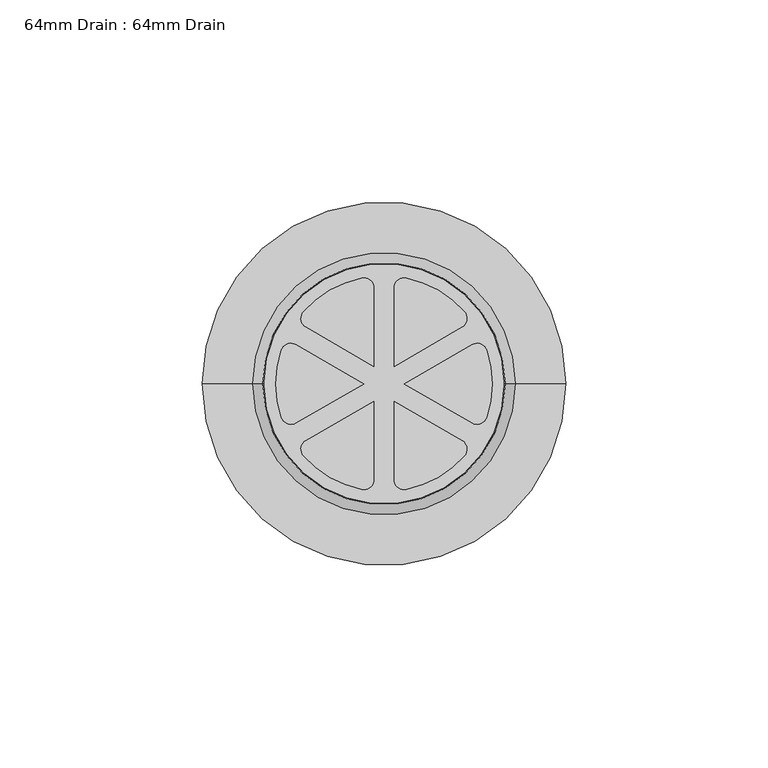
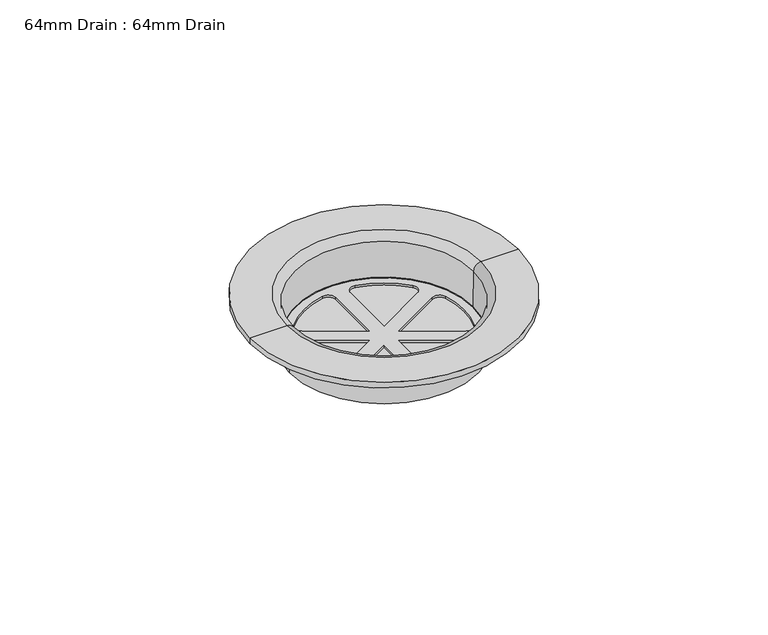
"""IFC4 building model written with IfcOpenShell, lengths in millimetres: flow terminal geometry, 64mm Drain : 64mm Drain."""

from ifc_helpers import new_model, si_unit, point, frame, frame_2d, origin, place, context, project, spatial, polyline, circle_curve, ellipse_curve, trimmed, segment, composite_curve, outline, extrude, source, transform, mapped, element, save
from ifc_brep_helpers import plane_surface, cylinder_surface, revolved_surface, advanced_brep


def flow_terminal_64mm_drain_64mm_drain_371441a0(model_context):
    return source(origin(), model_context, "Body", "SolidModel", [
        extrude(outline(composite_curve([segment(trimmed(circle_curve(frame_2d((-147.5947471, 0.0)), 29.738174), [point((-177.3329211, 0.0))], [point((-117.8565731, 0.0))], False, "CARTESIAN"), True, "CONTINUOUS"), segment(trimmed(circle_curve(frame_2d((-147.5947471, 0.0)), 29.738174), [point((-117.8565731, 0.0))], [point((-177.3329211, 0.0))], False, "CARTESIAN"), True, "CONTINUOUS")], self_intersect=False)), frame((0.0, 0.0, -15.0), z_axis=(0.0, 0.0, 1.0), x_axis=(1.0, 0.0, 0.0)), (0.0, 0.0, 1.0), 1.0),
        advanced_brep(
        [(-115.138004, 0.0, 2.0), (-180.0514903, 0.0, 2.0), (-177.551871, 0.0, -0.456369), (-117.6376232, 0.0, -0.456369), (-102.5947471, 0.0, 2.0), (-192.5947471, 0.0, 2.0), (-102.5947471, 0.0, 0.0), (-192.5947471, 0.0, 0.0), (-115.6293526, 0.0, 0.0), (-179.5601416, 0.0, 0.0), (-115.8911786, 0.0, -15.0), (-179.2983157, 0.0, -15.0), (-117.8565731, 0.0, -15.0), (-177.3329211, 0.0, -15.0), (-117.8565731, 0.0, -13.0), (-177.3329211, 0.0, -13.0)],
        [
            (0, 1, circle_curve(frame((-147.5947471, 0.0, 2.0), z_axis=(0.0, 0.0, 1.0), x_axis=(-1.0, 0.0, 0.0)), 32.4567432)),
            (1, 2, circle_curve(frame((-180.0514903, 0.0, -0.5), z_axis=(0.0, 1.0, 0.0), x_axis=(0.0, 0.0, 1.0)), 2.5)),
            (2, 3, circle_curve(frame((-147.5947471, 0.0, -0.456369), z_axis=(0.0, 0.0, -1.0), x_axis=(-1.0, 0.0, 0.0)), 29.9571239)),
            (3, 0, circle_curve(frame((-115.138004, 0.0, -0.5), z_axis=(0.0, 1.0, 0.0), x_axis=(0.0, 0.0, 1.0)), 2.5)),
            (1, 0, circle_curve(frame((-147.5947471, 0.0, 2.0), z_axis=(0.0, 0.0, 1.0), x_axis=(-1.0, 0.0, 0.0)), 32.4567432)),
            (3, 2, circle_curve(frame((-147.5947471, 0.0, -0.456369), z_axis=(0.0, 0.0, -1.0), x_axis=(-1.0, 0.0, 0.0)), 29.9571239)),
            (4, 5, circle_curve(frame((-147.5947471, 0.0, 2.0), z_axis=(0.0, 0.0, 1.0), x_axis=(-1.0, 0.0, 0.0)), 45.0)),
            (5, 1),
            (0, 4),
            (5, 4, circle_curve(frame((-147.5947471, 0.0, 2.0), z_axis=(0.0, 0.0, 1.0), x_axis=(-1.0, 0.0, 0.0)), 45.0)),
            (6, 7, circle_curve(frame((-147.5947471, 0.0, 0.0), z_axis=(0.0, 0.0, 1.0), x_axis=(-1.0, 0.0, 0.0)), 45.0)),
            (7, 5),
            (4, 6),
            (7, 6, circle_curve(frame((-147.5947471, 0.0, 0.0), z_axis=(0.0, 0.0, 1.0), x_axis=(-1.0, 0.0, 0.0)), 45.0)),
            (8, 9, circle_curve(frame((-147.5947471, 0.0, 0.0), z_axis=(0.0, 0.0, 1.0), x_axis=(-1.0, 0.0, 0.0)), 31.9653945)),
            (9, 7),
            (6, 8),
            (9, 8, circle_curve(frame((-147.5947471, 0.0, 0.0), z_axis=(0.0, 0.0, 1.0), x_axis=(-1.0, 0.0, 0.0)), 31.9653945)),
            (10, 11, circle_curve(frame((-147.5947471, 0.0, -15.0), z_axis=(0.0, 0.0, 1.0), x_axis=(-1.0, 0.0, 0.0)), 31.7035686)),
            (11, 9),
            (8, 10),
            (11, 10, circle_curve(frame((-147.5947471, 0.0, -15.0), z_axis=(0.0, 0.0, 1.0), x_axis=(-1.0, 0.0, 0.0)), 31.7035686)),
            (12, 13, circle_curve(frame((-147.5947471, 0.0, -15.0), z_axis=(0.0, 0.0, 1.0), x_axis=(-1.0, 0.0, 0.0)), 29.738174)),
            (13, 11),
            (10, 12),
            (13, 12, circle_curve(frame((-147.5947471, 0.0, -15.0), z_axis=(0.0, 0.0, 1.0), x_axis=(-1.0, 0.0, 0.0)), 29.738174)),
            (14, 15, circle_curve(frame((-147.5947471, 0.0, -13.0), z_axis=(0.0, 0.0, 1.0), x_axis=(-1.0, 0.0, 0.0)), 29.738174)),
            (15, 13),
            (12, 14),
            (15, 14, circle_curve(frame((-147.5947471, 0.0, -13.0), z_axis=(0.0, 0.0, 1.0), x_axis=(-1.0, 0.0, 0.0)), 29.738174)),
            (2, 15),
            (14, 3),
        ],
        [
            revolved_surface(trimmed(ellipse_curve(frame((-180.0514903, 0.0, -0.5), z_axis=(0.0, -1.0, 0.0), x_axis=(0.0, 0.0, 1.0)), 2.5, 2.5), [point((-177.551871, 0.0, -0.456369))], [point((-180.0514903, 0.0, 2.0))], True, "CARTESIAN"), (-147.5947471, 0.0, -523.0), (0.0, 0.0, -1.0)),
            plane_surface(frame((-147.5947471, 0.0, 2.0), z_axis=(0.0, 0.0, 1.0), x_axis=(-1.0, 0.0, 0.0))),
            cylinder_surface(frame((-147.5947471, 0.0, -523.0), z_axis=(0.0, 0.0, -1.0), x_axis=(-1.0, 0.0, 0.0)), 45.0),
            plane_surface(frame((-147.5947471, 0.0, 0.0), z_axis=(0.0, 0.0, -1.0), x_axis=(-1.0, 0.0, 0.0))),
            revolved_surface(polyline([(-179.5601416, 0.0, 0.0), (-179.2983157, 0.0, -15.0)]), (-147.5947471, 0.0, -523.0), (0.0, 0.0, -1.0)),
            plane_surface(frame((-147.5947471, 0.0, -15.0), z_axis=(0.0, 0.0, -1.0), x_axis=(-1.0, 0.0, 0.0))),
            revolved_surface(polyline([(-177.33292110000002, 0.0, -15.0), (-177.33292110000002, 0.0, -13.0)]), (-147.5947471, 0.0, -523.0), (0.0, 0.0, -1.0)),
            revolved_surface(polyline([(-177.3329211, 0.0, -13.0), (-177.551871, 0.0, -0.456369)]), (-147.5947471, 0.0, -523.0), (0.0, 0.0, -1.0)),
        ],
        [
            (0, [[1, 2, 3, 4]]),
            (0, [[5, -4, 6, -2]]),
            (1, [[7, 8, -1, 9]]),
            (1, [[10, -9, -5, -8]]),
            (2, [[11, 12, -7, 13]]),
            (2, [[14, -13, -10, -12]]),
            (3, [[15, 16, -11, 17]]),
            (3, [[18, -17, -14, -16]]),
            (4, [[19, 20, -15, 21]]),
            (4, [[22, -21, -18, -20]]),
            (5, [[23, 24, -19, 25]]),
            (5, [[26, -25, -22, -24]]),
            (6, [[27, 28, -23, 29]]),
            (6, [[30, -29, -26, -28]]),
            (7, [[-3, 31, -27, 32]]),
            (7, [[-6, -32, -30, -31]]),
        ],
    ),
        extrude(outline(composite_curve([segment(trimmed(circle_curve(frame_2d((-147.5947471, 0.0)), 29.738174), [point((-117.8565731, 0.0))], [point((-177.3329211, 0.0))], False, "CARTESIAN"), True, "CONTINUOUS"), segment(trimmed(circle_curve(frame_2d((-147.5947471, 0.0)), 29.738174), [point((-177.3329211, 0.0))], [point((-117.8565731, 0.0))], False, "CARTESIAN"), True, "CONTINUOUS")], self_intersect=False), holes=[composite_curve([segment(trimmed(circle_curve(frame_2d((-147.5947471, 0.0)), 26.738174), [point((-127.6947116, 17.8582904))], [point((-142.0790317, 26.1630815))], True, "CARTESIAN"), True, "CONTINUOUS"), segment(trimmed(circle_curve(frame_2d((-142.5947471, 23.7168522)), 2.5), [point((-142.0790317, 26.1630815))], [point((-145.0947471, 23.7168522))], True, "CARTESIAN"), True, "CONTINUOUS"), segment(polyline([(-145.0947471, 23.7168522), (-145.0947471, 4.330127), (-128.3053506, 14.0234896)]), True, "CONTINUOUS"), segment(trimmed(circle_curve(frame_2d((-129.5553506, 16.1885531)), 2.5), [point((-128.3053506, 14.0234896))], [point((-127.6947116, 17.8582904))], True, "CARTESIAN"), True, "CONTINUOUS")], self_intersect=False), composite_curve([segment(trimmed(circle_curve(frame_2d((-147.5947471, 0.0)), 26.738174), [point((-153.1104625, 26.1630815))], [point((-167.4947826, 17.8582904))], True, "CARTESIAN"), True, "CONTINUOUS"), segment(trimmed(circle_curve(frame_2d((-165.6341436, 16.1885531)), 2.5), [point((-167.4947826, 17.8582904))], [point((-166.8841436, 14.0234896))], True, "CARTESIAN"), True, "CONTINUOUS"), segment(polyline([(-166.8841436, 14.0234896), (-150.0947471, 4.330127), (-150.0947471, 23.7168522)]), True, "CONTINUOUS"), segment(trimmed(circle_curve(frame_2d((-152.5947471, 23.7168522)), 2.5), [point((-150.0947471, 23.7168522))], [point((-153.1104625, 26.1630815))], True, "CARTESIAN"), True, "CONTINUOUS")], self_intersect=False), composite_curve([segment(polyline([(-152.5947471, 0.0), (-169.3841436, 9.6933626)]), True, "CONTINUOUS"), segment(trimmed(circle_curve(frame_2d((-170.6341436, 7.5282991)), 2.5), [point((-169.3841436, 9.6933626))], [point((-173.010498, 8.3047911))], True, "CARTESIAN"), True, "CONTINUOUS"), segment(trimmed(circle_curve(frame_2d((-147.5947471, 0.0)), 26.738174), [point((-173.010498, 8.3047911))], [point((-173.010498, -8.3047911))], True, "CARTESIAN"), True, "CONTINUOUS"), segment(trimmed(circle_curve(frame_2d((-170.6341436, -7.5282991)), 2.5), [point((-173.010498, -8.3047911))], [point((-169.3841436, -9.6933626))], True, "CARTESIAN"), True, "CONTINUOUS"), segment(polyline([(-169.3841436, -9.6933626), (-152.5947471, 0.0)]), True, "CONTINUOUS")], self_intersect=False), composite_curve([segment(polyline([(-150.0947471, -4.330127), (-166.8841436, -14.0234896)]), True, "CONTINUOUS"), segment(trimmed(circle_curve(frame_2d((-165.6341436, -16.1885531)), 2.5), [point((-166.8841436, -14.0234896))], [point((-167.4947826, -17.8582904))], True, "CARTESIAN"), True, "CONTINUOUS"), segment(trimmed(circle_curve(frame_2d((-147.5947471, 0.0)), 26.738174), [point((-167.4947826, -17.8582904))], [point((-153.1104625, -26.1630815))], True, "CARTESIAN"), True, "CONTINUOUS"), segment(trimmed(circle_curve(frame_2d((-152.5947471, -23.7168522)), 2.5), [point((-153.1104625, -26.1630815))], [point((-150.0947471, -23.7168522))], True, "CARTESIAN"), True, "CONTINUOUS"), segment(polyline([(-150.0947471, -23.7168522), (-150.0947471, -4.330127)]), True, "CONTINUOUS")], self_intersect=False), composite_curve([segment(trimmed(circle_curve(frame_2d((-142.5947471, -23.7168522)), 2.5), [point((-145.0947471, -23.7168522))], [point((-142.0790317, -26.1630815))], True, "CARTESIAN"), True, "CONTINUOUS"), segment(trimmed(circle_curve(frame_2d((-147.5947471, 0.0)), 26.738174), [point((-142.0790317, -26.1630815))], [point((-127.6947116, -17.8582904))], True, "CARTESIAN"), True, "CONTINUOUS"), segment(trimmed(circle_curve(frame_2d((-129.5553506, -16.1885531)), 2.5), [point((-127.6947116, -17.8582904))], [point((-128.3053506, -14.0234896))], True, "CARTESIAN"), True, "CONTINUOUS"), segment(polyline([(-128.3053506, -14.0234896), (-145.0947471, -4.330127), (-145.0947471, -23.7168522)]), True, "CONTINUOUS")], self_intersect=False), composite_curve([segment(polyline([(-142.5947471, 0.0), (-125.8053506, -9.6933626)]), True, "CONTINUOUS"), segment(trimmed(circle_curve(frame_2d((-124.5553506, -7.5282991)), 2.5), [point((-125.8053506, -9.6933626))], [point((-122.1789962, -8.3047911))], True, "CARTESIAN"), True, "CONTINUOUS"), segment(trimmed(circle_curve(frame_2d((-147.5947471, 0.0)), 26.738174), [point((-122.1789962, -8.3047911))], [point((-122.1789962, 8.3047911))], True, "CARTESIAN"), True, "CONTINUOUS"), segment(trimmed(circle_curve(frame_2d((-124.5553506, 7.5282991)), 2.5), [point((-122.1789962, 8.3047911))], [point((-125.8053506, 9.6933626))], True, "CARTESIAN"), True, "CONTINUOUS"), segment(polyline([(-125.8053506, 9.6933626), (-142.5947471, 0.0)]), True, "CONTINUOUS")], self_intersect=False)]), frame((0.0, 0.0, -15.0), z_axis=(0.0, 0.0, 1.0), x_axis=(1.0, 0.0, 0.0)), (0.0, 0.0, 1.0), 2.0),
    ])


if __name__ == "__main__":
    model = new_model("IFC4")
    model_context = context("Model", 3, world=origin())
    ifc_project = project(units=[si_unit("LENGTHUNIT", "METRE", prefix="MILLI")], contexts=[model_context])
    site = spatial("IfcSite", under=ifc_project)
    building = spatial("IfcBuilding", under=site)
    placement = place(None, origin())
    flow_terminal_64mm_drain_64mm_drain_shape = flow_terminal_64mm_drain_64mm_drain_371441a0(model_context)
    element("IfcFlowTerminal", 1, ObjectType="64mm Drain : 64mm Drain", at=placement, inside=building, context=model_context, shape_type="MappedRepresentation", body=[
        mapped(flow_terminal_64mm_drain_64mm_drain_shape, transform((0.0, 0.0, 0.0), x_axis=(1.0, 0.0, 0.0), y_axis=(0.0, 1.0, 0.0), z_axis=(0.0, 0.0, 1.0))),
    ])
    save(model, "model.ifc")

# Revit data of these elements
# Type "64mm Drain : 64mm Drain"
#   Finish = none
#   Default Elevation = 0
#   Assembly Code = ""
# Element 1 (IfcFlowTerminal, "64mm Drain : 64mm Drain")
#   Materials on its faces: "Polished Chrome"
# Materials
#   "Polished Chrome": colour RGB 247 247 247, transparency 0
